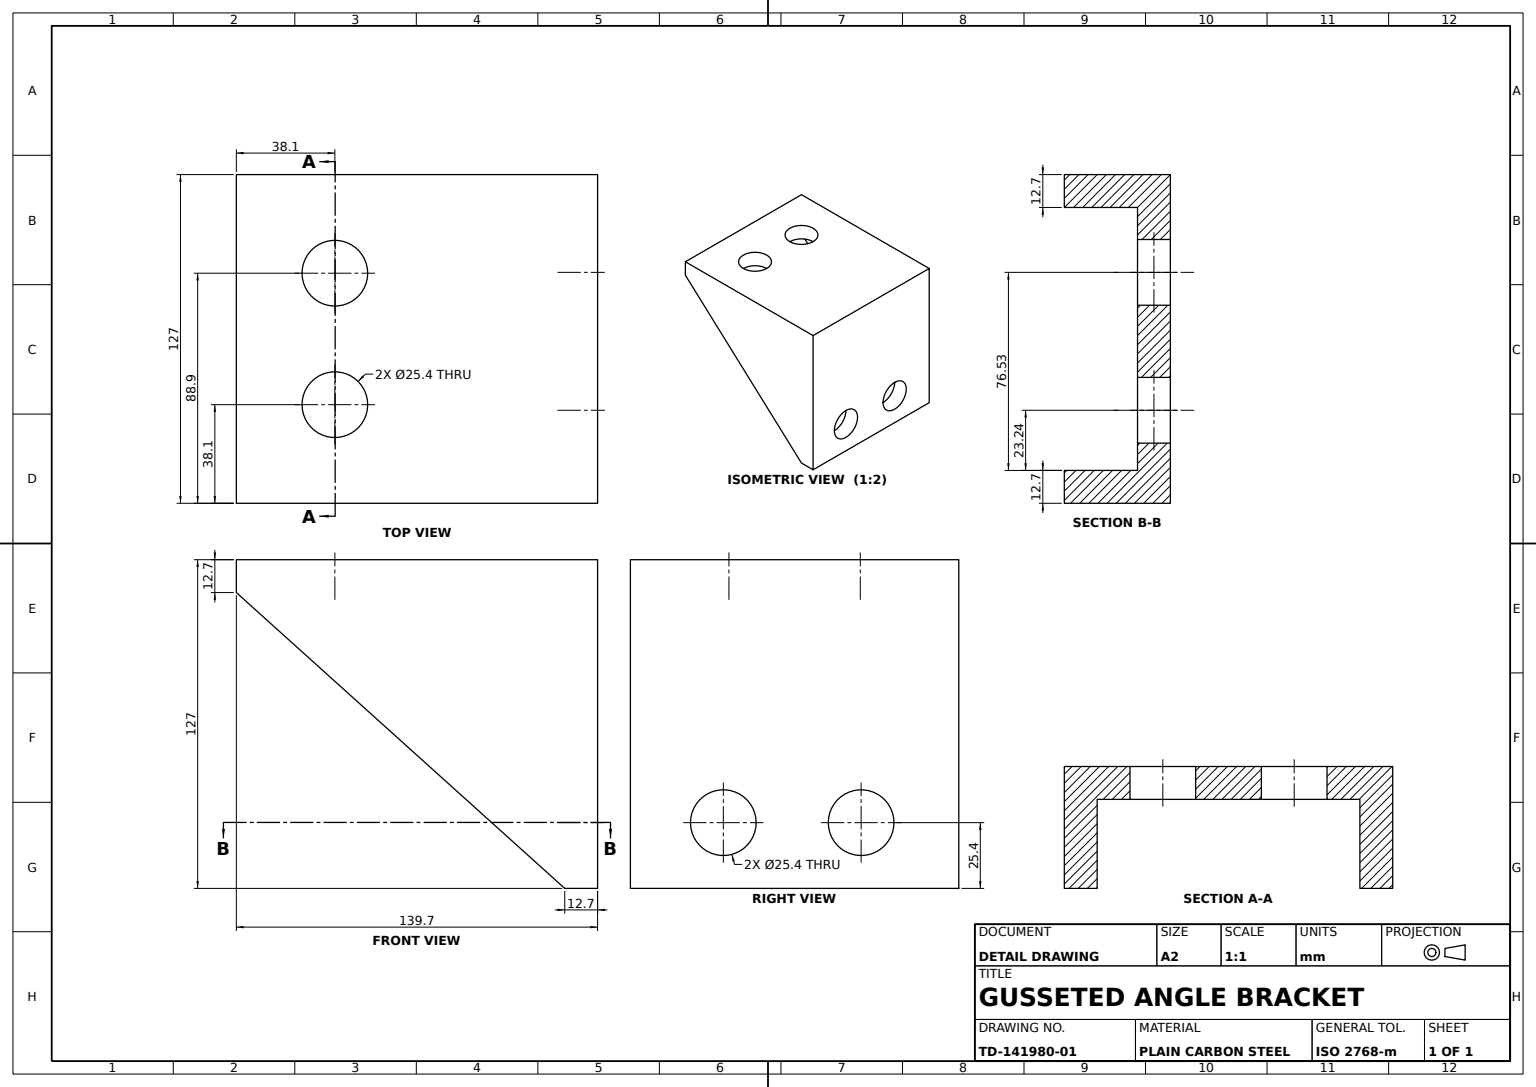
from build123d import *

# Parameters (mm, degrees)
BASE_PLATE_SKETCH_W      = 127
BASE_PLATE_SKETCH_H      = 127
BASE_PLATE_DEPTH         = 12.7
UPRIGHT_WALL_SKETCH_W    = 127
UPRIGHT_WALL_SKETCH_H    = 12.7
UPRIGHT_WALL_DEPTH       = 127
GUSSET_1_DEPTH           = 12.7
GUSSET_2_DEPTH           = 12.7
MOUNTING_HOLE_1_SKETCH_R = 12.7
MOUNTING_HOLE_1_DEPTH    = 12.7
MOUNTING_HOLE_2_SKETCH_R = 12.7
MOUNTING_HOLE_2_DEPTH    = 12.7
MOUNTING_HOLE_3_SKETCH_R = 12.7
MOUNTING_HOLE_3_DEPTH    = 12.7
MOUNTING_HOLE_4_SKETCH_R = 12.7
MOUNTING_HOLE_4_DEPTH    = 12.7


with BuildPart() as part:
    # Base Plate Sketch → Base Plate (new body)
    with BuildSketch(Plane.XY):
        with Locations((63.5, 63.5)):
            Rectangle(BASE_PLATE_SKETCH_W, BASE_PLATE_SKETCH_H)
    extrude(amount=BASE_PLATE_DEPTH)

    # Upright Wall Sketch → Upright Wall (add)
    with BuildSketch(Plane.XY.offset(12.7)):
        with Locations((63.5, 120.65)):
            Rectangle(UPRIGHT_WALL_SKETCH_W, UPRIGHT_WALL_SKETCH_H)
    extrude(amount=UPRIGHT_WALL_DEPTH)

    # Gusset 1 Sketch → Gusset 1 (add)
    with BuildSketch(Plane.ZY):
        Polygon((12.7, 0), (139.7, 114.3), (12.7, 114.3), align=None)
    extrude(amount=-GUSSET_1_DEPTH)

    # Gusset 2 Sketch → Gusset 2 (add)
    with BuildSketch(Plane(origin=(127, 0, 0), x_dir=(0, 0, -1), z_dir=(1, 0, 0))):
        Polygon((-12.7, 0), (-12.7, 114.3), (-139.7, 114.3), align=None)
    extrude(amount=-GUSSET_2_DEPTH)

    # Mounting Hole 1 Sketch → Mounting Hole 1 (cut)
    with BuildSketch(Plane.XZ.offset(-114.3)):
        with Locations(Location((38.1, 101.6, 0), (0, 0, 270))):
            Circle(MOUNTING_HOLE_1_SKETCH_R)
    extrude(amount=-MOUNTING_HOLE_1_DEPTH, mode=Mode.SUBTRACT)

    # Mounting Hole 2 Sketch → Mounting Hole 2 (cut)
    with BuildSketch(Plane.XZ.offset(-114.3)):
        with Locations(Location((88.9, 101.6, 0), (0, 0, 270))):
            Circle(MOUNTING_HOLE_2_SKETCH_R)
    extrude(amount=-MOUNTING_HOLE_2_DEPTH, mode=Mode.SUBTRACT)

    # Mounting Hole 3 Sketch → Mounting Hole 3 (cut)
    with BuildSketch(Plane.XY.offset(12.7)):
        with Locations((37.774003387, 25.4)):
            Circle(MOUNTING_HOLE_3_SKETCH_R)
    extrude(amount=-MOUNTING_HOLE_3_DEPTH, mode=Mode.SUBTRACT)

    # Mounting Hole 4 Sketch → Mounting Hole 4 (cut)
    with BuildSketch(Plane.XY.offset(12.7)):
        with Locations((91.0635678, 25.4)):
            Circle(MOUNTING_HOLE_4_SKETCH_R)
    extrude(amount=-MOUNTING_HOLE_4_DEPTH, mode=Mode.SUBTRACT)


solid = part.part
